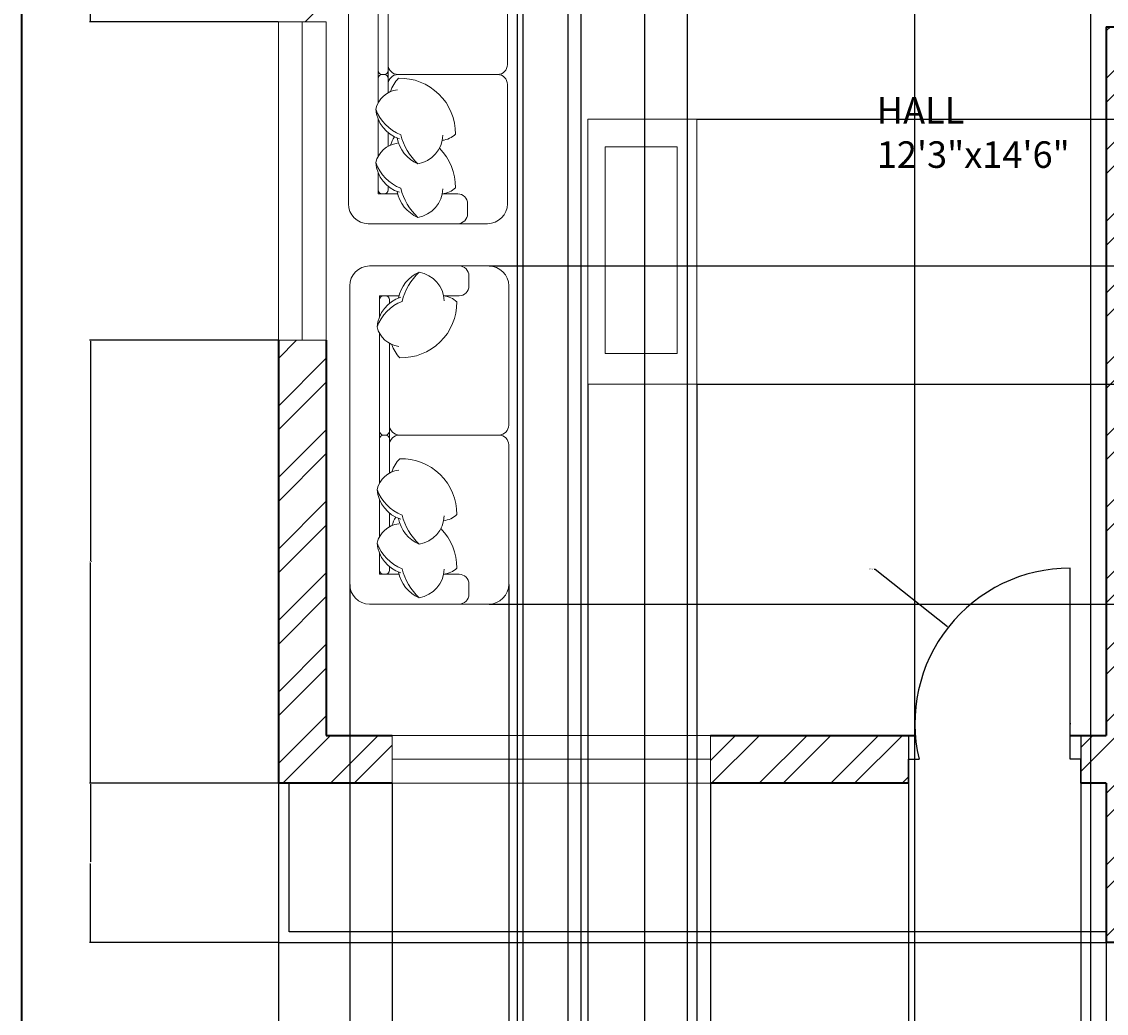
# Model space of a CAD drawing. Units: inches. Extents: x 2529 to 3014, y 1203 to 2262.
# Tile 2 of 13: x 2529 to 2733, y 1560 to 1747. Entities that reach past the tile are written whole.
import ezdxf

# ---------------------------------------------------------------- set-up
doc = ezdxf.new("R2010")
doc.units = ezdxf.units.IN
for name, color, linetype, lineweight in [('A-ANNO-DIMS', 2, 'Continuous', 18), ('A-ANNO-TTLB', 7, 'Continuous', 35), ('A-AREA-IDEN', 7, 'Continuous', 18), ('A-DOOR', 21, 'Continuous', 25), ('A-FLOR-RAIL', 61, 'Continuous', 25), ('A-FURN', 8, 'Continuous', 18), ('A-GLAZ', 191, 'Continuous', 18), ('A-WALL', 7, 'Continuous', 35), ('A-WALL-PATT', 143, 'Continuous', 13)]:
    doc.layers.add(name, color=color, linetype=linetype, lineweight=lineweight)
doc.styles.get("Standard").update_dxf_attribs({"font": 'arial.ttf'})
doc.dimstyles.get("Standard").update_dxf_attribs({"dimtxt": 0.18, "dimasz": 0.18, "dimexe": 0.18, "dimexo": 0.0625, "dimgap": 0.09, "dimtad": 0, "dimtih": 1, "dimtoh": 1, "dimdec": 4, "dimzin": 0, "dimdsep": 46, "dimtxsty": 'Standard', "dimcen": 0.09, "dimadec": 0, "dimazin": 0, "dimtfac": 1, "dimtdec": 4, "dimtofl": 0, "dimtmove": 0, "dimatfit": 3, "dimfxl": 1, "dimtolj": 1, "dimtzin": 0, "dimarcsym": 0})

# ---------------------------------------------------------------- blocks, each defined once
blk = doc.blocks.new('WIN-60x9')
for p, q in [((0, 60), (9, 60)), ((0, 60), (0, 0)), ((9, 60), (4.5, 60)), ((4.5, 60), (4.5, 0)), ((9, 60), (9, 0)), ((4.5, 0), (0, 0)), ((0, 0), (9, 0))]:
    blk.add_line(p, q)
blk = doc.blocks.new('*D18')
at = {"layer": 'A-ANNO-DIMS', "color": 0, "lineweight": -2, "transparency": 16777216}
for p, q in [((2577.06, 1573.44), (2577.06, 1483.77)), ((2733.06, 1573.44), (2733.06, 1483.77)), ((2577.24, 1483.95), (2654.78, 1483.95)), ((2732.88, 1483.95), (2655.34, 1483.95))]:
    blk.add_line(p, q, dxfattribs=at)
at = {"layer": 'A-ANNO-DIMS', "color": 0, "transparency": 16777216}
for points in [[(2577.24, 1483.98), (2577.24, 1483.92), (2577.06, 1483.95)], [(2732.88, 1483.98), (2732.88, 1483.92), (2733.06, 1483.95)]]:
    blk.add_solid(points, dxfattribs=at)
at = {"layer": 'Defpoints', "color": 0, "transparency": 16777216}
for p in [(2577.06, 1573.5), (2733.06, 1573.5), (2733.06, 1483.95)]:
    blk.add_point(p, dxfattribs=at)
at = {"layer": 'A-ANNO-DIMS', "color": 0, "transparency": 16777216, "insert": (2655.06, 1483.95), "char_height": 0.18, "attachment_point": 5}
blk.add_mtext('\\A1;156', dxfattribs=at)
blk = doc.blocks.new('*D19')
at = {"layer": 'A-ANNO-DIMS', "color": 0, "lineweight": -2, "transparency": 16777216}
for p, q in [((2839.56, 1582.44), (2839.56, 1483.77)), ((2733.06, 1573.44), (2733.06, 1483.77)), ((2733.24, 1483.95), (2785.92, 1483.95)), ((2839.38, 1483.95), (2786.69, 1483.95))]:
    blk.add_line(p, q, dxfattribs=at)
at = {"layer": 'A-ANNO-DIMS', "color": 0, "transparency": 16777216}
for points in [[(2733.24, 1483.98), (2733.24, 1483.92), (2733.06, 1483.95)], [(2839.38, 1483.98), (2839.38, 1483.92), (2839.56, 1483.95)]]:
    blk.add_solid(points, dxfattribs=at)
at = {"layer": 'Defpoints', "color": 0, "transparency": 16777216}
for p in [(2839.56, 1582.5), (2733.06, 1573.5), (2839.56, 1483.95)]:
    blk.add_point(p, dxfattribs=at)
at = {"layer": 'A-ANNO-DIMS', "color": 0, "transparency": 16777216, "insert": (2786.31, 1483.95), "char_height": 0.18, "attachment_point": 5}
blk.add_mtext('\\A1;106.5', dxfattribs=at)
blk = doc.blocks.new('*D21')
at = {"layer": 'A-ANNO-DIMS', "color": 0, "lineweight": -2, "transparency": 16777216}
for p, q in [((2576.99, 1603.5), (2541.45, 1603.5)), ((2541.63, 1603.32), (2541.63, 1588.69)), ((2541.63, 1573.68), (2541.63, 1588.32)), ((2576.99, 1573.5), (2541.45, 1573.5))]:
    blk.add_line(p, q, dxfattribs=at)
at = {"layer": 'A-ANNO-DIMS', "color": 0, "transparency": 16777216}
for points in [[(2541.6, 1603.32), (2541.66, 1603.32), (2541.63, 1603.5)], [(2541.6, 1573.68), (2541.66, 1573.68), (2541.63, 1573.5)]]:
    blk.add_solid(points, dxfattribs=at)
at = {"layer": 'Defpoints', "color": 0, "transparency": 16777216}
for p in [(2541.63, 1603.5), (2577.06, 1603.5), (2577.06, 1573.5)]:
    blk.add_point(p, dxfattribs=at)
at = {"layer": 'A-ANNO-DIMS', "color": 0, "transparency": 16777216, "insert": (2541.63, 1588.5), "char_height": 0.18, "attachment_point": 5}
blk.add_mtext('\\A1;30', dxfattribs=at)
blk = doc.blocks.new('*D22')
at = {"layer": 'A-ANNO-DIMS', "color": 0, "lineweight": -2, "transparency": 16777216}
for p, q in [((2576.99, 1686.95), (2541.45, 1686.95)), ((2541.63, 1686.77), (2541.63, 1645.41)), ((2541.63, 1603.68), (2541.63, 1645.04)), ((2576.99, 1603.5), (2541.45, 1603.5))]:
    blk.add_line(p, q, dxfattribs=at)
at = {"layer": 'A-ANNO-DIMS', "color": 0, "transparency": 16777216}
for points in [[(2541.6, 1686.77), (2541.66, 1686.77), (2541.63, 1686.95)], [(2541.6, 1603.68), (2541.66, 1603.68), (2541.63, 1603.5)]]:
    blk.add_solid(points, dxfattribs=at)
at = {"layer": 'Defpoints', "color": 0, "transparency": 16777216}
for p in [(2541.63, 1686.95), (2577.06, 1686.95), (2577.06, 1603.5)]:
    blk.add_point(p, dxfattribs=at)
at = {"layer": 'A-ANNO-DIMS', "color": 0, "transparency": 16777216, "insert": (2541.63, 1645.23), "char_height": 0.18, "attachment_point": 5}
blk.add_mtext('\\A1;83.45', dxfattribs=at)
blk = doc.blocks.new('*D23')
at = {"layer": 'A-ANNO-DIMS', "color": 0, "lineweight": -2, "transparency": 16777216}
for p, q in [((2585.99, 1791), (2541.45, 1791)), ((2541.63, 1790.82), (2541.63, 1769.16)), ((2541.63, 1747.13), (2541.63, 1768.79)), ((2576.99, 1746.95), (2541.45, 1746.95))]:
    blk.add_line(p, q, dxfattribs=at)
at = {"layer": 'A-ANNO-DIMS', "color": 0, "transparency": 16777216}
for points in [[(2541.6, 1790.82), (2541.66, 1790.82), (2541.63, 1791)], [(2541.6, 1747.13), (2541.66, 1747.13), (2541.63, 1746.95)]]:
    blk.add_solid(points, dxfattribs=at)
at = {"layer": 'Defpoints', "color": 0, "transparency": 16777216}
for p in [(2541.63, 1791), (2586.06, 1791), (2577.06, 1746.95)]:
    blk.add_point(p, dxfattribs=at)
at = {"layer": 'A-ANNO-DIMS', "color": 0, "transparency": 16777216, "insert": (2541.63, 1768.98), "char_height": 0.18, "attachment_point": 5}
blk.add_mtext('\\A1;44.055', dxfattribs=at)
blk = doc.blocks.new('*D33')
at = {"layer": 'A-ANNO-DIMS', "color": 0, "lineweight": -2, "transparency": 16777216}
for p, q in [((2577.06, 1603.44), (2577.06, 1483.77)), ((2598.48, 1603.44), (2598.48, 1483.77)), ((2577.24, 1483.95), (2587.37, 1483.95)), ((2598.3, 1483.95), (2588.16, 1483.95))]:
    blk.add_line(p, q, dxfattribs=at)
at = {"layer": 'A-ANNO-DIMS', "color": 0, "transparency": 16777216}
for points in [[(2577.24, 1483.98), (2577.24, 1483.92), (2577.06, 1483.95)], [(2598.3, 1483.98), (2598.3, 1483.92), (2598.48, 1483.95)]]:
    blk.add_solid(points, dxfattribs=at)
at = {"layer": 'Defpoints', "color": 0, "transparency": 16777216}
for p in [(2577.06, 1603.5), (2598.48, 1603.5), (2598.48, 1483.95)]:
    blk.add_point(p, dxfattribs=at)
at = {"layer": 'A-ANNO-DIMS', "color": 0, "transparency": 16777216, "insert": (2587.77, 1483.95), "char_height": 0.18, "attachment_point": 5}
blk.add_mtext('\\A1;21.42', dxfattribs=at)
blk = doc.blocks.new('*D34')
at = {"layer": 'A-ANNO-DIMS', "color": 0, "lineweight": -2, "transparency": 16777216}
for p, q in [((2658.48, 1603.44), (2658.48, 1483.77)), ((2695.77, 1603.44), (2695.77, 1483.77)), ((2658.66, 1483.95), (2676.73, 1483.95)), ((2695.59, 1483.95), (2677.52, 1483.95))]:
    blk.add_line(p, q, dxfattribs=at)
at = {"layer": 'A-ANNO-DIMS', "color": 0, "transparency": 16777216}
for points in [[(2658.66, 1483.98), (2658.66, 1483.92), (2658.48, 1483.95)], [(2695.59, 1483.98), (2695.59, 1483.92), (2695.77, 1483.95)]]:
    blk.add_solid(points, dxfattribs=at)
at = {"layer": 'Defpoints', "color": 0, "transparency": 16777216}
for p in [(2658.48, 1603.5), (2695.77, 1603.5), (2695.77, 1483.95)]:
    blk.add_point(p, dxfattribs=at)
at = {"layer": 'A-ANNO-DIMS', "color": 0, "transparency": 16777216, "insert": (2677.12, 1483.95), "char_height": 0.18, "attachment_point": 5}
blk.add_mtext('\\A1;37.29', dxfattribs=at)
blk = doc.blocks.new('*D35')
at = {"layer": 'A-ANNO-DIMS', "color": 0, "lineweight": -2, "transparency": 16777216}
for p, q in [((2695.77, 1603.44), (2695.77, 1483.77)), ((2728.25, 1603.44), (2728.25, 1483.77)), ((2695.95, 1483.95), (2711.61, 1483.95)), ((2728.07, 1483.95), (2712.4, 1483.95))]:
    blk.add_line(p, q, dxfattribs=at)
at = {"layer": 'A-ANNO-DIMS', "color": 0, "transparency": 16777216}
for points in [[(2695.95, 1483.98), (2695.95, 1483.92), (2695.77, 1483.95)], [(2728.07, 1483.98), (2728.07, 1483.92), (2728.25, 1483.95)]]:
    blk.add_solid(points, dxfattribs=at)
at = {"layer": 'Defpoints', "color": 0, "transparency": 16777216}
for p in [(2695.77, 1603.5), (2728.25, 1603.5), (2728.25, 1483.95)]:
    blk.add_point(p, dxfattribs=at)
at = {"layer": 'A-ANNO-DIMS', "color": 0, "transparency": 16777216, "insert": (2712.01, 1483.95), "char_height": 0.18, "attachment_point": 5}
blk.add_mtext('\\A1;32.48', dxfattribs=at)
blk = doc.blocks.new('*D42')
at = {"layer": 'A-ANNO-DIMS', "color": 0, "lineweight": -2, "transparency": 16777216}
for p, q in [((2590.48, 1640.92), (2590.48, 1483.77)), ((2620.46, 1640.92), (2620.46, 1483.77)), ((2590.66, 1483.95), (2605.07, 1483.95)), ((2620.28, 1483.95), (2605.86, 1483.95))]:
    blk.add_line(p, q, dxfattribs=at)
at = {"layer": 'A-ANNO-DIMS', "color": 0, "transparency": 16777216}
for points in [[(2590.66, 1483.98), (2590.66, 1483.92), (2590.48, 1483.95)], [(2620.28, 1483.98), (2620.28, 1483.92), (2620.46, 1483.95)]]:
    blk.add_solid(points, dxfattribs=at)
at = {"layer": 'Defpoints', "color": 0, "transparency": 16777216}
for p in [(2590.48, 1640.98), (2620.46, 1640.98), (2620.46, 1483.95)]:
    blk.add_point(p, dxfattribs=at)
at = {"layer": 'A-ANNO-DIMS', "color": 0, "transparency": 16777216, "insert": (2605.47, 1483.95), "char_height": 0.18, "attachment_point": 5}
blk.add_mtext('\\A1;29.98', dxfattribs=at)
blk = doc.blocks.new('*D43')
at = {"layer": 'A-ANNO-DIMS', "color": 0, "lineweight": -2, "transparency": 16777216}
for p, q in [((2616.77, 1700.93), (3007.66, 1700.93)), ((3007.48, 1700.75), (3007.48, 1669.26)), ((3007.48, 1637.41), (3007.48, 1668.9)), ((2616.77, 1637.23), (3007.66, 1637.23))]:
    blk.add_line(p, q, dxfattribs=at)
at = {"layer": 'A-ANNO-DIMS', "color": 0, "transparency": 16777216}
for points in [[(3007.45, 1700.75), (3007.51, 1700.75), (3007.48, 1700.93)], [(3007.45, 1637.41), (3007.51, 1637.41), (3007.48, 1637.23)]]:
    blk.add_solid(points, dxfattribs=at)
at = {"layer": 'Defpoints', "color": 0, "transparency": 16777216}
for p in [(2616.71, 1700.93), (3007.48, 1700.93), (2616.71, 1637.23)]:
    blk.add_point(p, dxfattribs=at)
at = {"layer": 'A-ANNO-DIMS', "color": 0, "transparency": 16777216, "insert": (3007.48, 1669.08), "char_height": 0.18, "attachment_point": 5}
blk.add_mtext('\\A1;63.7', dxfattribs=at)
blk = doc.blocks.new('*D44')
at = {"layer": 'A-ANNO-DIMS', "color": 0, "lineweight": -2, "transparency": 16777216}
for p, q in [((2635.37, 1678.62), (2635.37, 1483.77)), ((2655.89, 1678.62), (2655.89, 1483.77)), ((2635.55, 1483.95), (2645.17, 1483.95)), ((2655.71, 1483.95), (2646.1, 1483.95))]:
    blk.add_line(p, q, dxfattribs=at)
at = {"layer": 'A-ANNO-DIMS', "color": 0, "transparency": 16777216}
for points in [[(2635.55, 1483.98), (2635.55, 1483.92), (2635.37, 1483.95)], [(2655.71, 1483.98), (2655.71, 1483.92), (2655.89, 1483.95)]]:
    blk.add_solid(points, dxfattribs=at)
at = {"layer": 'Defpoints', "color": 0, "transparency": 16777216}
for p in [(2635.37, 1678.68), (2655.89, 1678.68), (2655.89, 1483.95)]:
    blk.add_point(p, dxfattribs=at)
at = {"layer": 'A-ANNO-DIMS', "color": 0, "transparency": 16777216, "insert": (2645.63, 1483.95), "char_height": 0.18, "attachment_point": 5}
blk.add_mtext('\\A1;20.517', dxfattribs=at)
blk = doc.blocks.new('*D45')
at = {"layer": 'A-ANNO-DIMS', "color": 0, "lineweight": -2, "transparency": 16777216}
for p, q in [((2655.95, 1728.6), (3007.66, 1728.6)), ((3007.48, 1728.42), (3007.48, 1703.82)), ((3007.48, 1678.86), (3007.48, 1703.46)), ((2655.95, 1678.68), (3007.66, 1678.68))]:
    blk.add_line(p, q, dxfattribs=at)
at = {"layer": 'A-ANNO-DIMS', "color": 0, "transparency": 16777216}
for points in [[(3007.45, 1728.42), (3007.51, 1728.42), (3007.48, 1728.6)], [(3007.45, 1678.86), (3007.51, 1678.86), (3007.48, 1678.68)]]:
    blk.add_solid(points, dxfattribs=at)
at = {"layer": 'Defpoints', "color": 0, "transparency": 16777216}
for p in [(2655.89, 1728.6), (3007.48, 1728.6), (2655.89, 1678.68)]:
    blk.add_point(p, dxfattribs=at)
at = {"layer": 'A-ANNO-DIMS', "color": 0, "transparency": 16777216, "insert": (3007.48, 1703.64), "char_height": 0.18, "attachment_point": 5}
blk.add_mtext('\\A1;49.92', dxfattribs=at)
blk = doc.blocks.new('*D53')
at = {"layer": 'A-ANNO-DIMS', "color": 0, "lineweight": -2, "transparency": 16777216}
for p, q in [((2696.93, 1790.94), (2696.93, 1483.77)), ((2730.09, 1790.94), (2730.09, 1483.77)), ((2697.11, 1483.95), (2713.11, 1483.95)), ((2729.91, 1483.95), (2713.9, 1483.95))]:
    blk.add_line(p, q, dxfattribs=at)
at = {"layer": 'A-ANNO-DIMS', "color": 0, "transparency": 16777216}
for points in [[(2697.11, 1483.98), (2697.11, 1483.92), (2696.93, 1483.95)], [(2729.91, 1483.98), (2729.91, 1483.92), (2730.09, 1483.95)]]:
    blk.add_solid(points, dxfattribs=at)
at = {"layer": 'Defpoints', "color": 0, "transparency": 16777216}
for p in [(2696.93, 1791), (2730.09, 1791), (2730.09, 1483.95)]:
    blk.add_point(p, dxfattribs=at)
at = {"layer": 'A-ANNO-DIMS', "color": 0, "transparency": 16777216, "insert": (2713.51, 1483.95), "char_height": 0.18, "attachment_point": 5}
blk.add_mtext('\\A1;33.15', dxfattribs=at)
blk = doc.blocks.new('*D65')
at = {"layer": 'A-ANNO-DIMS', "color": 0, "lineweight": -2, "transparency": 16777216}
for p, q in [((2646.06, 1874.24), (2646.06, 1483.77)), ((2654.06, 1874.24), (2654.06, 1483.77)), ((2646.24, 1483.95), (2649.91, 1483.95)), ((2653.88, 1483.95), (2650.2, 1483.95))]:
    blk.add_line(p, q, dxfattribs=at)
at = {"layer": 'A-ANNO-DIMS', "color": 0, "transparency": 16777216}
for points in [[(2646.24, 1483.98), (2646.24, 1483.92), (2646.06, 1483.95)], [(2653.88, 1483.98), (2653.88, 1483.92), (2654.06, 1483.95)]]:
    blk.add_solid(points, dxfattribs=at)
at = {"layer": 'Defpoints', "color": 0, "transparency": 16777216}
for p in [(2646.06, 1874.3), (2654.06, 1874.3), (2654.06, 1483.95)]:
    blk.add_point(p, dxfattribs=at)
at = {"layer": 'A-ANNO-DIMS', "color": 0, "transparency": 16777216, "insert": (2650.06, 1483.95), "char_height": 0.18, "attachment_point": 5}
blk.add_mtext('\\A1;8', dxfattribs=at)
blk = doc.blocks.new('*D71')
at = {"layer": 'A-ANNO-DIMS', "color": 0, "lineweight": -2, "transparency": 16777216}
for p, q in [((2623.09, 2159.68), (2623.09, 1483.77)), ((2631.58, 2159.68), (2631.58, 1483.77)), ((2623.27, 1483.95), (2626.94, 1483.95)), ((2631.4, 1483.95), (2627.73, 1483.95))]:
    blk.add_line(p, q, dxfattribs=at)
at = {"layer": 'A-ANNO-DIMS', "color": 0, "transparency": 16777216}
for points in [[(2623.27, 1483.98), (2623.27, 1483.92), (2623.09, 1483.95)], [(2631.4, 1483.98), (2631.4, 1483.92), (2631.58, 1483.95)]]:
    blk.add_solid(points, dxfattribs=at)
at = {"layer": 'Defpoints', "color": 0, "transparency": 16777216}
for p in [(2623.09, 2159.75), (2631.58, 2159.75), (2631.58, 1483.95)]:
    blk.add_point(p, dxfattribs=at)
at = {"layer": 'A-ANNO-DIMS', "color": 0, "transparency": 16777216, "insert": (2627.33, 1483.95), "char_height": 0.18, "attachment_point": 5}
blk.add_mtext('\\A1;8.484', dxfattribs=at)
blk = doc.blocks.new('*D74')
at = {"layer": 'A-ANNO-DIMS', "color": 0, "lineweight": -2, "transparency": 16777216}
for p, q in [((2622.06, 2135.91), (2622.06, 1483.77)), ((2634.06, 2135.91), (2634.06, 1483.77)), ((2622.24, 1483.95), (2627.6, 1483.95)), ((2633.88, 1483.95), (2628.51, 1483.95))]:
    blk.add_line(p, q, dxfattribs=at)
at = {"layer": 'A-ANNO-DIMS', "color": 0, "transparency": 16777216}
for points in [[(2622.24, 1483.98), (2622.24, 1483.92), (2622.06, 1483.95)], [(2633.88, 1483.98), (2633.88, 1483.92), (2634.06, 1483.95)]]:
    blk.add_solid(points, dxfattribs=at)
at = {"layer": 'Defpoints', "color": 0, "transparency": 16777216}
for p in [(2622.06, 2135.98), (2634.06, 2135.98), (2634.06, 1483.95)]:
    blk.add_point(p, dxfattribs=at)
at = {"layer": 'A-ANNO-DIMS', "color": 0, "transparency": 16777216, "insert": (2628.06, 1483.95), "char_height": 0.18, "attachment_point": 5}
blk.add_mtext('\\A1;12.002', dxfattribs=at)
blk = doc.blocks.new('*D84')
at = {"layer": 'A-ANNO-DIMS', "color": 0, "lineweight": -2, "transparency": 16777216}
for p, q in [((2689.34, 1643.79), (2689.52, 1643.79)), ((2689.52, 1643.79), (2703.15, 1633.01)), ((2726.16, 1614.74), (2726.34, 1614.74)), ((2726.25, 1614.65), (2726.25, 1614.83))]:
    blk.add_line(p, q, dxfattribs=at)
at = {"layer": 'A-ANNO-DIMS', "color": 0, "transparency": 16777216}
blk.add_solid([(2703.17, 1633.03), (2703.14, 1632.98), (2703.3, 1632.89)], dxfattribs=at)
at = {"layer": 'Defpoints', "color": 0, "transparency": 16777216}
for p in [(2703.3, 1632.89), (2726.25, 1614.74)]:
    blk.add_point(p, dxfattribs=at)
at = {"layer": 'A-ANNO-DIMS', "color": 0, "transparency": 16777216, "insert": (2688.79, 1643.79), "char_height": 0.18, "attachment_point": 5}
blk.add_mtext('\\A1;R29.266', dxfattribs=at)

msp = doc.modelspace()

# ---------------------------------------------------------------- hatches: boundary and pattern name
at = {"layer": 'A-WALL-PATT'}
h = msp.add_hatch(dxfattribs=at)
h.set_pattern_fill('ANSI32', color=256)
h.paths.add_polyline_path([(2686.5554, 2106.5032), (2622.0554, 2106.5032), (2622.0554, 2109.2964), (2617.4223, 2109.2964), (2613.0554, 2109.2964), (2613.0554, 2106.5032), (2577.0554, 2106.5032), (2577.0554, 2092.6918), (2586.0554, 2092.6918), (2586.0554, 2102.0032), (2682.0554, 2102.0032), (2682.0554, 2099.9833), (2686.5554, 2099.9833), (2686.5554, 2102.0032)])
h.paths.add_polyline_path([(2695.2249, 2054.0032), (2686.5554, 2054.0032), (2686.5554, 2080.2316), (2684.3054, 2080.2316), (2682.0554, 2080.2316), (2682.0554, 2054.0032), (2586.0554, 2054.0032), (2586.0554, 2068.6918), (2577.0554, 2068.6918), (2577.0554, 2019.1229), (2586.0554, 2019.1229), (2586.0554, 2049.5032), (2695.2249, 2049.5032)])
h.paths.add_polyline_path([(2737.5554, 2049.5032), (2866.5554, 2049.5032), (2866.5554, 2045.0233), (2871.0554, 2045.0233), (2871.0554, 2049.5032), (2871.0554, 2172.5032), (2866.5554, 2172.5032), (2829.1265, 2172.5032), (2829.1265, 2168.0032), (2866.5554, 2168.0032), (2866.5554, 2054.0032), (2737.5554, 2054.0032), (2737.5554, 2056.4892), (2735.3054, 2056.4892), (2733.0554, 2056.4892), (2733.0554, 2049.5032), (2733.0554, 1917.5032), (2733.0554, 1913.0032), (2871.0554, 1913.0032), (2871.0554, 1924.9149), (2868.8054, 1924.9149), (2866.5554, 1924.9149), (2866.5554, 1917.5032), (2737.5554, 1917.5032)], flags=17)
h.paths.add_polyline_path([(2972.0554, 2207.5032), (2613.0554, 2207.5032), (2613.0554, 2205.5032), (2613.0554, 2188.9366), (2622.0554, 2188.9366), (2622.0554, 2198.5032), (2733.0554, 2198.5032), (2733.0554, 2084.8053), (2735.3054, 2084.8053), (2737.5554, 2084.8053), (2737.5554, 2168.0032), (2769.1265, 2168.0032), (2769.1265, 2170.2532), (2769.1265, 2172.5032), (2737.5554, 2172.5032), (2737.5554, 2198.5032), (2963.0554, 2198.5032), (2963.0554, 2093.5032), (2912.0586, 2093.5032), (2912.0586, 2089.0032), (2918.5554, 2089.0032), (2918.5554, 2031.8749), (2923.0554, 2031.8749), (2923.0554, 2089.0032), (2963.0554, 2089.0032), (2963.0554, 2010.0032), (2923.0554, 2010.0032), (2923.0554, 2011.9417), (2918.5554, 2011.9417), (2918.5554, 2003.1338), (2923.0554, 2003.1338), (2923.0554, 2005.5032), (2963.0554, 2005.5032), (2963.0554, 1917.5032), (2963.0554, 1691.0776), (2972.0554, 1691.0776), (2972.0554, 1917.5032)])
h.paths.add_polyline_path([(2963.0554, 1945.5032), (2923.0554, 1945.5032), (2923.0554, 1983.0571), (2920.8054, 1983.0571), (2918.5554, 1983.0571), (2918.5554, 1941.0032), (2963.0554, 1941.0032)], flags=17)
h.paths.add_polyline_path([(2930.3679, 1788.7532), (2930.3679, 1791.0032), (2894.8637, 1791.0032), (2894.8637, 1786.5032), (2900.5554, 1786.5032), (2900.5554, 1784.6931), (2905.0554, 1784.6931), (2905.0554, 1786.5032), (2930.3679, 1786.5032)], flags=17)
h.paths.add_polyline_path([(2963.0554, 1791.0032), (2954.3679, 1791.0032), (2954.3679, 1786.5032), (2963.0554, 1786.5032)], flags=17)
h.paths.add_polyline_path([(2871.0554, 1853.0032), (2919.0554, 1853.0032), (2919.0554, 1847.0972), (2923.5554, 1847.0972), (2923.5554, 1853.0032), (2923.5554, 1857.5032), (2871.0554, 1857.5032), (2871.0554, 1871.7024), (2866.5554, 1871.7024), (2866.5554, 1791.0032), (2737.5554, 1791.0032), (2737.5554, 1806.6712), (2735.3054, 1806.6712), (2733.0554, 1806.6712), (2733.0554, 1791.0032), (2733.0554, 1786.5032), (2733.0554, 1780.6235), (2737.5554, 1780.6235), (2737.5554, 1786.5032), (2872.8745, 1786.5032), (2872.8745, 1788.7532), (2872.8745, 1791.0032), (2871.0554, 1791.0032)], flags=17)
h.paths.add_polyline_path([(2844.0554, 1734.0032), (2848.2652, 1734.0032), (2848.2652, 1738.5032), (2800.0167, 1738.5032), (2800.0167, 1734.0032), (2839.5554, 1734.0032), (2839.5554, 1582.5032), (2792.3334, 1582.5032), (2792.3334, 1573.5032), (2871.4433, 1573.5032), (2871.4433, 1578.0032), (2871.4433, 1582.5032), (2844.0554, 1582.5032)])
h.paths.add_polyline_path([(2972.0554, 1631.0776), (2963.0554, 1631.0776), (2963.0554, 1582.5032), (2931.4433, 1582.5032), (2931.4433, 1573.5032), (2972.0554, 1573.5032)])
h.paths.add_polyline_path([(2756.3334, 1582.5032), (2737.5554, 1582.5032), (2737.5554, 1734.0032), (2744.3201, 1734.0032), (2744.3201, 1738.5032), (2737.5554, 1738.5032), (2737.5554, 1746.0094), (2733.0554, 1746.0094), (2733.0554, 1738.5032), (2733.0554, 1612.5032), (2728.2475, 1612.5032), (2728.2475, 1603.5032), (2733.0554, 1603.5032), (2733.0554, 1582.5032), (2733.0554, 1573.5032), (2756.3334, 1573.5032), (2756.3334, 1578.0032)])
h.paths.add_polyline_path([(2695.7662, 1612.5032), (2658.4771, 1612.5032), (2658.4771, 1603.5032), (2695.7662, 1603.5032), (2695.7662, 1608.0032)])
h.paths.add_polyline_path([(2586.0554, 1686.9483), (2577.0554, 1686.9483), (2577.0554, 1603.5032), (2598.4771, 1603.5032), (2598.4771, 1608.0032), (2598.4771, 1612.5032), (2586.0554, 1612.5032)])
h.paths.add_polyline_path([(2683.2727, 1791.0032), (2586.0554, 1791.0032), (2586.0554, 1815.6736), (2581.5554, 1815.6736), (2577.0554, 1815.6736), (2577.0554, 1746.9483), (2586.0554, 1746.9483), (2586.0554, 1786.5032), (2683.2727, 1786.5032)])
h.paths.add_polyline_path([(2586.0554, 1959.1229), (2577.0554, 1959.1229), (2577.0554, 1875.6736), (2586.0554, 1875.6736), (2586.0554, 1913.0032), (2683.2727, 1913.0032), (2683.2727, 1917.5032), (2586.0554, 1917.5032)])

# ---------------------------------------------------------------- linework, layer by layer
at = {"layer": 'A-ANNO-TTLB'}
msp.add_lwpolyline([(2528.6765, 2261.8165), (3013.6003, 2261.8165), (3013.6003, 1455.1523), (2528.6765, 1455.1523)], close=True, dxfattribs=at)
at = {"layer": 'A-DOOR'}
for p, q in [((2726.2475, 1608.0032), (2726.2475, 1644.0032)), ((2695.7662, 1612.5032), (2695.7662, 1603.5032)), ((2728.2475, 1612.5032), (2728.2475, 1603.5032)), ((2695.7662, 1603.5032), (2695.7662, 1608.0032)), ((2695.7662, 1608.0032), (2697.7662, 1608.0032)), ((2728.2475, 1608.0032), (2726.2475, 1608.0032)), ((2728.2475, 1603.5032), (2728.2475, 1608.0032))]:
    msp.add_line(p, q, dxfattribs=at)
msp.add_arc((2726.2475, 1614.7368), 29.2664, 90, 193.30178, dxfattribs=at)
at = {"layer": 'A-FLOR-RAIL'}
for p, q in [((2577.0554, 1603.5032), (2577.0554, 1573.5032)), ((2579.0554, 1575.5032), (2579.0554, 1603.5032)), ((2733.0554, 1575.5032), (2579.0554, 1575.5032)), ((2733.0554, 1573.5032), (2733.0554, 1575.5032)), ((2577.0554, 1573.5032), (2733.0554, 1573.5032))]:
    msp.add_line(p, q, dxfattribs=at)
at = {"layer": 'A-FURN', "ltscale": 0.03}
for points in [[(2620.206, 1738.8743, -0.41421356), (2618.3324, 1737.0007, -0.41421356), (2620.206, 1735.1271), (2620.206, 1712.6442, -0.41421356), (2616.4588, 1708.897), (2593.9759, 1708.897, -0.41421356), (2590.2287, 1712.6442), (2590.2287, 1761.3573, -0.41421356), (2593.9759, 1765.1045), (2616.4588, 1765.1045, -0.41421356), (2620.206, 1761.3573), (2620.206, 1738.8743, -0.41421356), (2618.3324, 1737.0007, -0.41421356), (2620.206, 1735.1271)], [(2620.4577, 1670.956, -0.41421356), (2618.5841, 1669.0824, -0.41421356), (2620.4577, 1667.2088), (2620.4577, 1640.9787, -0.41421356), (2616.7105, 1637.2315), (2594.2276, 1637.2315, -0.41421356), (2590.4804, 1640.9787), (2590.4804, 1697.1861, -0.41421356), (2594.2276, 1700.9333), (2616.7105, 1700.9333, -0.41421356), (2620.4577, 1697.1861), (2620.4577, 1670.956, -0.41421356), (2618.5841, 1669.0824, -0.41421356), (2620.4577, 1667.2088)]]:
    msp.add_lwpolyline(points, format="xyb", dxfattribs=at)
at = {"layer": 'A-FURN'}
for points in [[(2595.8494, 1752.4253), (2595.8494, 1731.6691)], [(2595.8494, 1728.5522), (2595.8494, 1721.5762)], [(2599.7832, 1695.3126), (2596.1011, 1695.3126), (2596.1011, 1691.3711)], [(2596.1011, 1688.2541), (2596.1011, 1660.0036)], [(2596.1011, 1656.8867), (2596.1011, 1649.9107)]]:
    msp.add_lwpolyline(points, dxfattribs=at)
for points in [[(2595.8494, 1752.4253), (2595.8494, 1737.7502, 0.41421356), (2596.5989, 1737.0007), (2596.9736, 1737.0007, 0.41421356), (2597.723, 1737.7502), (2597.723, 1750.5387, 0.41421356)], [(2597.723, 1738.8743, 0.41421356), (2599.5966, 1737.0007)], [(2597.723, 1738.8743, 0.41421356), (2599.5966, 1737.0007), (2618.3324, 1737.0007, 0.41421356)], [(2595.8494, 1731.6691), (2595.8494, 1736.2513, -0.41421356), (2596.5989, 1737.0007), (2596.9736, 1737.0007, -0.41421356), (2597.723, 1736.2513), (2597.723, 1733.5557, -0.41421356)], [(2597.723, 1735.1271, -0.41421356), (2599.5966, 1737.0007)], [(2597.723, 1735.1271, -0.41421356), (2599.5966, 1737.0007), (2618.3324, 1737.0007, -0.41421356)], [(2607.9344, 1724.6066, 0.16554063), (2610.4099, 1725.7656, 0.42598917), (2599.6768, 1736.288, 0.12152332), (2598.1974, 1733.7902, -7.11546429)], [(2599.8495, 1724.9018, -0.30666349), (2595.3835, 1730.49, -0.30632997), (2599.4621, 1734.1406, 0.87284716)], [(2603.326, 1720.1823, -0.14772988), (2600.1061, 1725.6583, -0.21334276), (2595.3835, 1730.49, -0.17866181)], [(2595.8494, 1721.5762), (2595.8494, 1728.5522, -0.41421356)], [(2597.723, 1726.0404), (2597.723, 1723.4628, -0.41421356)], [(2598.9299, 1725.2681, 0.07186538), (2598.1974, 1723.6973, -7.11546429)], [(2608.0486, 1725.5509, -0.35677236), (2603.326, 1720.1823, -0.24954205), (2599.4342, 1725.0467, 9.61688035)], [(2599.8495, 1714.8088, -0.30666349), (2595.3835, 1720.3971, -0.30632997), (2599.4621, 1724.0477, 0.87284716)], [(2607.9344, 1714.5137, 0.16554063), (2610.4099, 1715.6727, 0.20023115), (2607.395, 1723.1102, 0.12152332)], [(2603.326, 1710.0894, -0.14772988), (2600.1061, 1715.5654, -0.21334276), (2595.3835, 1720.3971, -0.17866181)], [(2595.8494, 1715.2672), (2595.8494, 1718.4592, -0.41421356)], [(2595.8494, 1718.4592), (2595.8494, 1714.5177), (2599.5315, 1714.5177, -0.41421356)], [(2597.723, 1715.9475), (2597.723, 1715.2672, -0.41421356), (2596.9736, 1714.5177), (2596.5989, 1714.5177, -0.41421356), (2595.8494, 1715.2672)], [(2608.0486, 1715.458, -0.35677236), (2603.326, 1710.0894, -0.24954205), (2599.4342, 1714.9538, 9.61688035)], [(2607.9352, 1714.5177), (2610.8381, 1714.5177, -0.41421356), (2612.7117, 1712.6442), (2612.7117, 1710.7706, -0.41421356), (2610.8381, 1708.897)], [(2611.0898, 1700.9333, -0.41421356), (2612.9634, 1699.0597), (2612.9634, 1697.1861, -0.41421356), (2611.0898, 1695.3126), (2608.1869, 1695.3126)], [(2603.5777, 1699.7409, 0.14772988), (2600.3578, 1694.265, 0.21334276), (2595.6352, 1689.4332, 0.17866181)], [(2608.3003, 1694.3723, 0.35677236), (2603.5777, 1699.7409, 0.24954205), (2599.6859, 1694.8765, -9.61688035)], [(2600.1012, 1695.0215, 0.30666349), (2595.6352, 1689.4332, 0.30632997), (2599.7138, 1685.7826, -0.87284716)], [(2597.9747, 1693.8828), (2597.9747, 1694.5631, 0.41421356), (2597.2253, 1695.3126), (2596.8506, 1695.3126, 0.41421356), (2596.1011, 1694.5631)], [(2596.1011, 1694.5631), (2596.1011, 1691.3711, 0.41421356)], [(2608.1861, 1695.3166, -0.16554063), (2610.6616, 1694.1576, -0.42598917), (2599.9285, 1683.6352, -0.12152332), (2598.4491, 1686.133, 7.11546429)], [(2596.1011, 1688.2541), (2596.1011, 1669.8319, 0.41421356), (2596.8506, 1669.0824), (2597.2253, 1669.0824, 0.41421356), (2597.9747, 1669.8319), (2597.9747, 1686.3675, 0.41421356)], [(2597.9747, 1670.956, 0.41421356), (2599.8483, 1669.0824)], [(2597.9747, 1670.956, 0.41421356), (2599.8483, 1669.0824), (2618.5841, 1669.0824, 0.41421356)], [(2596.1011, 1660.0036), (2596.1011, 1668.333, -0.41421356), (2596.8506, 1669.0824), (2597.2253, 1669.0824, -0.41421356), (2597.9747, 1668.333), (2597.9747, 1661.8902, -0.41421356)], [(2597.9747, 1667.2088, -0.41421356), (2599.8483, 1669.0824)], [(2597.9747, 1667.2088, -0.41421356), (2599.8483, 1669.0824), (2618.5841, 1669.0824, -0.41421356)], [(2608.1861, 1652.9411, 0.16554063), (2610.6616, 1654.1002, 0.42598917), (2599.9285, 1664.6226, 0.12152332), (2598.4491, 1662.1248, -7.11546429)], [(2600.1012, 1653.2363, -0.30666349), (2595.6352, 1658.8245, -0.30632997), (2599.7138, 1662.4751, 0.87284716)], [(2603.5777, 1648.5169, -0.14772988), (2600.3578, 1653.9928, -0.21334276), (2595.6352, 1658.8245, -0.17866181)], [(2596.1011, 1649.9107), (2596.1011, 1656.8867, -0.41421356)], [(2597.9747, 1654.3749), (2597.9747, 1651.7973, -0.41421356)], [(2599.1816, 1653.6026, 0.07186538), (2598.4491, 1652.0318, -7.11546429)], [(2608.3003, 1653.8854, -0.35677236), (2603.5777, 1648.5169, -0.24954205), (2599.6859, 1653.3813, 9.61688035)], [(2600.1012, 1643.1434, -0.30666349), (2595.6352, 1648.7316, -0.30632997), (2599.7138, 1652.3822, 0.87284716)], [(2608.1861, 1642.8482, 0.16554063), (2610.6616, 1644.0073, 0.20023115), (2607.6467, 1651.4447, 0.12152332)], [(2603.5777, 1638.4239, -0.14772988), (2600.3578, 1643.8999, -0.21334276), (2595.6352, 1648.7316, -0.17866181)], [(2596.1011, 1646.7938), (2596.1011, 1642.8523), (2599.7832, 1642.8523, -0.41421356)], [(2596.1011, 1643.6017), (2596.1011, 1646.7938, -0.41421356)], [(2597.9747, 1644.282), (2597.9747, 1643.6017, -0.41421356), (2597.2253, 1642.8523), (2596.8506, 1642.8523, -0.41421356), (2596.1011, 1643.6017)], [(2608.3003, 1643.7925, -0.35677236), (2603.5777, 1638.4239, -0.24954205), (2599.6859, 1643.2884, 9.61688035)], [(2608.1869, 1642.8523), (2611.0898, 1642.8523, -0.41421356), (2612.9634, 1640.9787), (2612.9634, 1639.1051, -0.41421356), (2611.0898, 1637.2315)]]:
    msp.add_lwpolyline(points, format="xyb", dxfattribs=at)
for points in [[(2595.8494, 1737.7502), (2595.8494, 1736.2513, -0.41421356), (2596.5989, 1737.0007), (2596.9736, 1737.0007, -0.41421356), (2597.723, 1736.2513), (2597.723, 1737.7502, -0.41421356), (2596.9736, 1737.0007), (2596.5989, 1737.0007, -0.41421356)], [(2596.1011, 1669.8319), (2596.1011, 1668.333, -0.41421356), (2596.8506, 1669.0824), (2597.2253, 1669.0824, -0.41421356), (2597.9747, 1668.333), (2597.9747, 1669.8319, -0.41421356), (2597.2253, 1669.0824), (2596.8506, 1669.0824, -0.41421356)]]:
    msp.add_lwpolyline(points, format="xyb", close=True, dxfattribs=at)
for points in [[(2635.3732, 1728.5992), (2655.8904, 1728.5992), (2655.8904, 1678.6815), (2635.3732, 1678.6815)], [(2638.6428, 1723.354), (2652.1593, 1723.354), (2652.1593, 1684.4155), (2638.6428, 1684.4155)]]:
    msp.add_lwpolyline(points, close=True, dxfattribs=at)
at = {"layer": 'A-WALL'}
for p, q in [((2733.0554, 1746.0094), (2737.5554, 1746.0094)), ((2733.0554, 1746.0094), (2733.0554, 1738.5032)), ((2733.0554, 1738.5032), (2733.0554, 1612.5032)), ((2577.0554, 1686.9483), (2577.0554, 1603.5032)), ((2586.0554, 1686.9483), (2586.0554, 1612.5032)), ((2586.0554, 1686.9483), (2586.0554, 1612.5032)), ((2586.0554, 1612.5032), (2598.4771, 1612.5032)), ((2658.4771, 1612.5032), (2697.0664, 1612.5032)), ((2726.2475, 1612.5032), (2733.0554, 1612.5032)), ((2598.4771, 1603.5032), (2577.0554, 1603.5032)), ((2695.7662, 1603.5032), (2658.4771, 1603.5032)), ((2733.0554, 1603.5032), (2728.2475, 1603.5032)), ((2733.0554, 1603.5032), (2733.0554, 1582.5032)), ((2733.0554, 1582.5032), (2733.0554, 1573.5032)), ((2756.3334, 1573.5032), (2733.0554, 1573.5032))]:
    msp.add_line(p, q, dxfattribs=at)

# ---------------------------------------------------------------- block references
at = {"layer": 'A-GLAZ'}
msp.add_blockref('WIN-60x9', (2577.055, 1686.9484), dxfattribs=at)
at = {"layer": 'A-GLAZ', "rotation": 90.00000000000261}
msp.add_blockref('WIN-60x9', (2658.477, 1603.5029), dxfattribs=at)

# ---------------------------------------------------------------- texts
at = {"layer": 'A-AREA-IDEN', "insert": (2689.8014, 1732.7448), "char_height": 5, "attachment_point": 1}
msp.add_mtext_dynamic_manual_height_columns('HALL\\P12\'3"x14\'6"', width=153.965463, gutter_width=12.5, heights=[0], dxfattribs=at)

# ---------------------------------------------------------------- dimensions: what is measured, and where the dimension line sits
at = {"layer": 'A-ANNO-DIMS'}
for base, p1, p2, override, picture, middle in [((2631.5753, 1483.9492), (2623.0916, 2159.7466), (2631.5753, 2159.7466), {"dimdec": 3, "dimlfac": 1, "dimrnd": 0, "dimzin": 0, "dimdsep": 46, "dimlunit": 2}, '*D71', (2627.3335, 1483.9492)), ((2634.0572, 1483.9492), (2622.0554, 2135.9767), (2634.0572, 2135.9767), {"dimdec": 3, "dimlfac": 1, "dimrnd": 0, "dimzin": 0, "dimdsep": 46, "dimlunit": 2}, '*D74', (2628.0563, 1483.9492)), ((2654.0554, 1483.9492), (2646.0554, 1874.3024), (2654.0554, 1874.3024), {"dimdec": 0, "dimlfac": 1, "dimrnd": 0, "dimzin": 0, "dimdsep": 46, "dimlunit": 2}, '*D65', (2650.0554, 1483.9492)), ((2730.085, 1483.9492), (2696.9325, 1791.0032), (2730.085, 1791.0032), {"dimdec": 2, "dimlfac": 1, "dimrnd": 0, "dimzin": 0, "dimdsep": 46, "dimlunit": 2}, '*D53', (2713.5087, 1483.9492)), ((2655.8904, 1483.9492), (2635.3732, 1678.6815), (2655.8904, 1678.6815), {"dimdec": 3, "dimlfac": 1, "dimrnd": 0, "dimzin": 0, "dimdsep": 46, "dimlunit": 2}, '*D44', (2645.6318, 1483.9492)), ((2620.4577, 1483.9492), (2590.4804, 1640.9787), (2620.4577, 1640.9787), {"dimdec": 2, "dimlfac": 1, "dimrnd": 0, "dimzin": 0, "dimdsep": 46, "dimlunit": 2}, '*D42', (2605.4691, 1483.9492)), ((2598.4771, 1483.9492), (2577.0554, 1603.5032), (2598.4771, 1603.5032), {"dimdec": 2, "dimlfac": 1, "dimrnd": 0, "dimzin": 0, "dimdsep": 46, "dimlunit": 2}, '*D33', (2587.7662, 1483.9492)), ((2695.7662, 1483.9492), (2658.4771, 1603.5032), (2695.7662, 1603.5032), {"dimdec": 2, "dimlfac": 1, "dimrnd": 0, "dimzin": 0, "dimdsep": 46, "dimlunit": 2}, '*D34', (2677.1217, 1483.9492)), ((2728.2475, 1483.9492), (2695.7662, 1603.5032), (2728.2475, 1603.5032), {"dimdec": 2, "dimlfac": 1, "dimrnd": 0, "dimzin": 0, "dimdsep": 46, "dimlunit": 2}, '*D35', (2712.0068, 1483.9492)), ((2839.5554, 1483.9492), (2733.0554, 1573.5032), (2839.5554, 1582.5032), {"dimdec": 1, "dimlfac": 1, "dimrnd": 0, "dimzin": 0, "dimdsep": 46, "dimlunit": 2}, '*D19', (2786.3054, 1483.9492)), ((2733.0554, 1483.9492), (2577.0554, 1573.5032), (2733.0554, 1573.5032), {"dimdec": 0, "dimlfac": 1, "dimrnd": 0, "dimzin": 0, "dimdsep": 46, "dimlunit": 2}, '*D18', (2655.0554, 1483.9492))]:
    dim = msp.add_linear_dim(base=base, p1=p1, p2=p2, dimstyle='Standard', override=override, dxfattribs=at)
    dim.commit()
    dim.dimension.update_dxf_attribs({"geometry": picture, "text_midpoint": middle})
for base, p1, p2, override, picture, middle in [((2541.6304, 1791.0032), (2577.0554, 1746.9483), (2586.0554, 1791.0032), {"dimdec": 3, "dimlfac": 1, "dimrnd": 0, "dimzin": 0, "dimdsep": 46, "dimlunit": 2}, '*D23', (2541.6304, 1768.9757)), ((3007.4804, 1728.5992), (2655.8904, 1678.6815), (2655.8904, 1728.5992), {"dimdec": 2, "dimlfac": 1, "dimrnd": 0, "dimzin": 0, "dimdsep": 46, "dimlunit": 2}, '*D45', (3007.4804, 1703.6403)), ((3007.4804, 1700.9333), (2616.7105, 1637.2315), (2616.7105, 1700.9333), {"dimdec": 1, "dimlfac": 1, "dimrnd": 0, "dimzin": 0, "dimdsep": 46, "dimlunit": 2}, '*D43', (3007.4804, 1669.0824)), ((2541.6304, 1686.9483), (2577.0554, 1603.5032), (2577.0554, 1686.9483), {"dimdec": 2, "dimlfac": 1, "dimrnd": 0, "dimzin": 0, "dimdsep": 46, "dimlunit": 2}, '*D22', (2541.6304, 1645.2257)), ((2541.6304, 1603.5032), (2577.0554, 1573.5032), (2577.0554, 1603.5032), {"dimdec": 0, "dimlfac": 1, "dimrnd": 0, "dimzin": 0, "dimdsep": 46, "dimlunit": 2}, '*D21', (2541.6304, 1588.5032))]:
    dim = msp.add_linear_dim(base=base, p1=p1, p2=p2, angle=90, dimstyle='Standard', override=override, dxfattribs=at)
    dim.commit()
    dim.dimension.update_dxf_attribs({"geometry": picture, "text_midpoint": middle})
dim = msp.add_radius_dim(center=(2726.2475, 1614.7368), mpoint=(2703.2952, 1632.8949), dimstyle='Standard', override={"dimdec": 3, "dimlfac": 1, "dimrnd": 0, "dimzin": 0, "dimdsep": 46, "dimlunit": 2}, dxfattribs=at)
dim.commit()
dim.dimension.update_dxf_attribs({"geometry": '*D84', "text_midpoint": (2688.7941, 1643.7897), "dimtype": 164})

doc.saveas('drawing.dxf')
